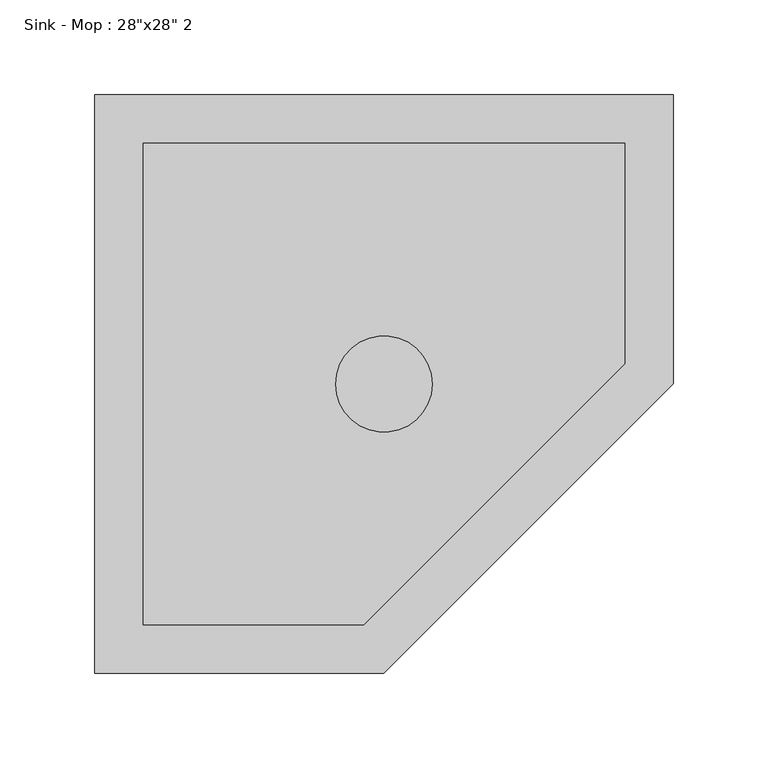
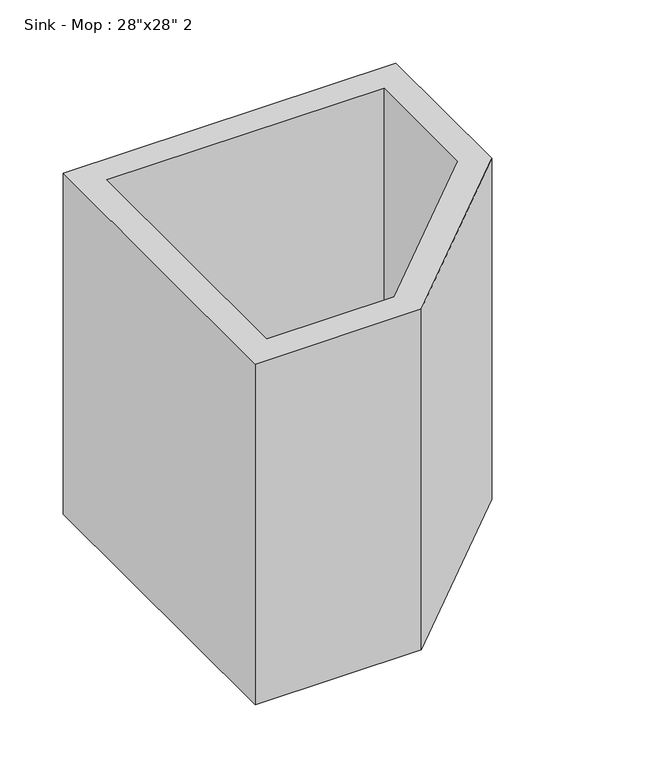
"""IFC4 building model written with IfcOpenShell, lengths in millimetres: flow terminal geometry."""

from ifc_helpers import new_model, si_unit, point, frame, frame_2d, origin, origin_with_axes, place, context, project, spatial, polyline, circle_curve, trimmed, segment, composite_curve, outline, extrude, source, transform, mapped, element, save
from ifc_brep_helpers import plane_surface, revolved_surface, advanced_brep


def flow_terminal_080557f2(model_context):
    return source(origin(), model_context, "Body", "SolidModel", [
        advanced_brep(
        [(304.8, 0.0, 330.2), (0.0, 0.0, 330.2), (0.0, -304.8, 330.2), (152.4, -304.8, 330.2), (304.8, -152.4, 330.2), (25.4, -25.4, 330.2), (279.4, -25.4, 330.2), (279.4, -141.8789755, 330.2), (141.8789755, -279.4, 330.2), (25.4, -279.4, 330.2), (304.8, 0.0, 0.0), (304.8, -152.4, 0.0), (152.4, -304.8, 0.0), (0.0, -304.8, 0.0), (0.0, 0.0, 0.0), (127.0, -152.4, 0.0), (177.8, -152.4, 0.0), (279.4, -25.4, 25.4), (25.4, -25.4, 25.4), (25.4, -279.4, 25.4), (141.8789755, -279.4, 25.4), (279.4, -141.8789755, 25.4), (177.8, -152.4, 25.4), (127.0, -152.4, 25.4)],
        [
            (0, 1),
            (1, 2),
            (2, 3),
            (3, 4),
            (4, 0),
            (5, 6),
            (6, 7),
            (7, 8),
            (8, 9),
            (9, 5),
            (10, 11),
            (11, 12),
            (12, 13),
            (13, 14),
            (14, 10),
            (15, 16, circle_curve(frame((152.4, -152.4, 0.0), z_axis=(0.0, 0.0, 1.0), x_axis=(1.0, 0.0, 0.0)), 25.4)),
            (16, 15, circle_curve(frame((152.4, -152.4, 0.0), z_axis=(0.0, 0.0, 1.0), x_axis=(1.0, 0.0, 0.0)), 25.4)),
            (0, 10),
            (14, 1),
            (13, 2),
            (12, 3),
            (11, 4),
            (17, 18),
            (18, 19),
            (19, 20),
            (20, 21),
            (21, 17),
            (22, 23, circle_curve(frame((152.4, -152.4, 25.4), z_axis=(0.0, 0.0, -1.0), x_axis=(1.0, 0.0, 0.0)), 25.4)),
            (23, 22, circle_curve(frame((152.4, -152.4, 25.4), z_axis=(0.0, 0.0, -1.0), x_axis=(1.0, 0.0, 0.0)), 25.4)),
            (17, 6),
            (5, 18),
            (9, 19),
            (8, 20),
            (7, 21),
            (22, 16),
            (15, 23),
        ],
        [
            plane_surface(frame((0.0, 0.0, 330.2), z_axis=(0.0, 0.0, 1.0), x_axis=(-1.0, 0.0, 0.0))),
            plane_surface(frame((0.0, 0.0, 0.0), z_axis=(0.0, 0.0, -1.0), x_axis=(1.0, 0.0, 0.0))),
            plane_surface(frame((304.8, 0.0, 330.2), z_axis=(0.0, 1.0, 0.0), x_axis=(0.0, 0.0, -1.0))),
            plane_surface(frame((0.0, 0.0, 330.2), z_axis=(-1.0, 0.0, 0.0), x_axis=(0.0, 0.0, -1.0))),
            plane_surface(frame((0.0, -304.8, 330.2), z_axis=(0.0, -1.0, 0.0), x_axis=(0.0, 0.0, -1.0))),
            plane_surface(frame((152.4, -304.8, 330.2), z_axis=(0.7071067811865438, -0.7071067811865512, 0.0), x_axis=(0.0, 0.0, -1.0))),
            plane_surface(frame((304.8, -152.4, 330.2), z_axis=(1.0, 0.0, 0.0), x_axis=(0.0, 0.0, -1.0))),
            plane_surface(frame((25.4, -25.4, 25.4), z_axis=(0.0, 0.0, 1.0), x_axis=(1.0, 0.0, 0.0))),
            plane_surface(frame((279.4, -25.4, 330.2), z_axis=(0.0, -1.0, 0.0), x_axis=(0.0, 0.0, -1.0))),
            plane_surface(frame((25.4, -25.4, 330.2), z_axis=(1.0, 0.0, 0.0), x_axis=(0.0, 0.0, -1.0))),
            plane_surface(frame((25.4, -279.4, 330.2), z_axis=(0.0, 1.0, 0.0), x_axis=(0.0, 0.0, -1.0))),
            plane_surface(frame((141.8789755, -279.4, 330.2), z_axis=(-0.7071067811865651, 0.70710678118653, 0.0), x_axis=(0.0, 0.0, -1.0))),
            plane_surface(frame((279.4, -141.8789755, 330.2), z_axis=(-1.0, 0.0, 0.0), x_axis=(0.0, 0.0, -1.0))),
            revolved_surface(polyline([(177.8, -152.4, 25.4), (177.8, -152.4, 0.0)]), (152.4, -152.4, 0.0), (0.0, 0.0, 1.0)),
        ],
        [
            (0, [[1, 2, 3, 4, 5], [6, 7, 8, 9, 10]]),
            (1, [[11, 12, 13, 14, 15], [16, 17]]),
            (2, [[-1, 18, -15, 19]]),
            (3, [[-2, -19, -14, 20]]),
            (4, [[-3, -20, -13, 21]]),
            (5, [[-4, -21, -12, 22]]),
            (6, [[-5, -22, -11, -18]]),
            (7, [[23, 24, 25, 26, 27], [28, 29]]),
            (8, [[-23, 30, -6, 31]]),
            (9, [[-24, -31, -10, 32]]),
            (10, [[-25, -32, -9, 33]]),
            (11, [[-26, -33, -8, 34]]),
            (12, [[-27, -34, -7, -30]]),
            (13, [[35, -16, 36, -28]]),
            (13, [[-35, -29, -36, -17]]),
        ],
    ),
        extrude(outline(composite_curve([segment(trimmed(circle_curve(frame_2d((152.4, -152.4)), 25.4), [point((127.0, -152.4))], [point((177.8, -152.4))], False, "CARTESIAN"), True, "CONTINUOUS"), segment(trimmed(circle_curve(frame_2d((152.4, -152.4)), 25.4), [point((177.8, -152.4))], [point((127.0, -152.4))], False, "CARTESIAN"), True, "CONTINUOUS")], self_intersect=False)), origin_with_axes(), (0.0, 0.0, 1.0), 25.4),
    ])


if __name__ == "__main__":
    model = new_model("IFC4")
    model_context = context("Model", 3, world=origin())
    ifc_project = project(units=[si_unit("LENGTHUNIT", "METRE", prefix="MILLI")], contexts=[model_context])
    site = spatial("IfcSite", under=ifc_project)
    building = spatial("IfcBuilding", under=site)
    placement = place(None, origin())
    flow_terminal_shape = flow_terminal_080557f2(model_context)
    element("IfcFlowTerminal", 1, ObjectType="Sink - Mop : 28\"x28\" 2", at=placement, inside=building, context=model_context, shape_type="MappedRepresentation", body=[
        mapped(flow_terminal_shape, transform((0.0, 0.0, 0.0), x_axis=(1.0, 0.0, 0.0), y_axis=(0.0, 1.0, 0.0), z_axis=(0.0, 0.0, 1.0))),
    ])
    save(model, "model.ifc")

# Revit data of these elements
# Type "Sink - Mop : 28\"x28\" 2"
#   WFU = 2
#   Sink Width = 1' - 0"
#   Sink Length = 1' - 0"
#   Sanitary Radius = 1"
#   Sanitary Diameter = 2"
#   Half Sink Width = 0' - 6"
#   Half Sink Length = 0' - 6"
#   Sink Material = none
#   HWFU = 0
#   Default Elevation = 0
#   CWFU = 0
#   Assembly Code = ""
